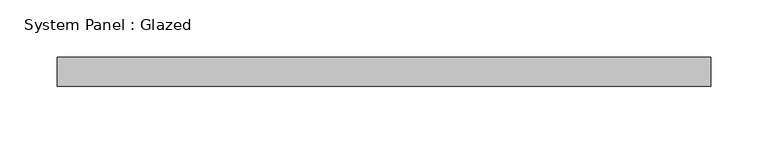
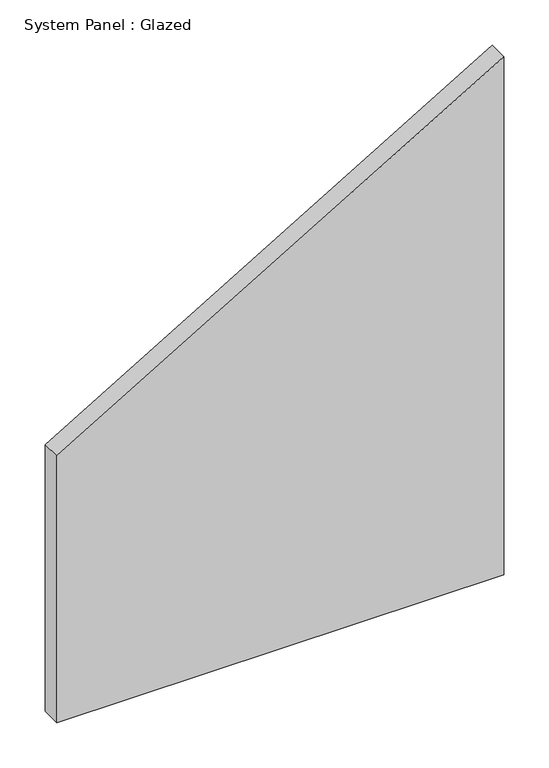
"""IFC4 building model written with IfcOpenShell, lengths in millimetres: plate geometry, System Panel : Glazed."""

from ifc_helpers import new_model, si_unit, frame, origin, place, context, project, spatial, polyline, outline, extrude, source, transform, mapped, element, save


def system_panel_glazed_0e80e67f(model_context):
    return source(origin(), model_context, "Body", "SweptSolid", [
        extrude(outline(polyline([(0.0, -285.75), (0.0, 285.75), (700.3109514, 285.75), (360.6432431, -285.75), (0.0, -285.75)])), frame((0.0, 19.05, 0.0), z_axis=(0.0, 1.0, 0.0), x_axis=(0.0, 0.0, 1.0)), (0.0, 0.0, 1.0), 25.4),
    ])


if __name__ == "__main__":
    model = new_model("IFC4")
    model_context = context("Model", 3, world=origin())
    ifc_project = project(units=[si_unit("LENGTHUNIT", "METRE", prefix="MILLI")], contexts=[model_context])
    site = spatial("IfcSite", under=ifc_project)
    building = spatial("IfcBuilding", under=site)
    placement = place(None, origin())
    system_panel_glazed_shape = system_panel_glazed_0e80e67f(model_context)
    element("IfcPlate", 1, ObjectType="System Panel : Glazed", at=placement, inside=building, context=model_context, shape_type="MappedRepresentation", body=[
        mapped(system_panel_glazed_shape, transform((0.0, 0.0, 0.0), x_axis=(1.0, 0.0, 0.0), y_axis=(0.0, 1.0, 0.0), z_axis=(0.0, 0.0, 1.0))),
    ])
    save(model, "model.ifc")

# Revit data of these elements
# Type "System Panel : Glazed"
#   Construction Type Id = "GSP4R"
#   Analytic Construction = "1/8 in Pilkington single glazing"
#   Visual Light Transmittance = 0.9
#   Solar Heat Gain Coefficient = 0.86
#   Heat Transfer Coefficient (U) = 1.18115 BTU/(h·ft²·°F)
#   Define Thermal Properties by = 1
# Element 1 (IfcPlate, "System Panel : Glazed")
#   Materials on its faces: "Glass"
# Materials
#   "Glass": class "Glass", colour RGB 0 128 192, transparency 0.75, Description = "Soda Lime Glass", Cost = 0
